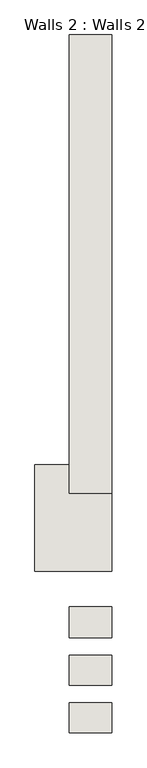
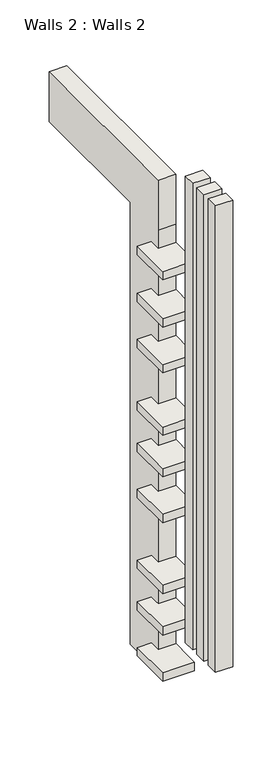
"""IFC4 building model written with IfcOpenShell, lengths in millimetres: wall geometry, Walls 2 : Walls 2."""

from ifc_helpers import new_model, si_unit, frame, origin, place, context, project, spatial, polyline, outline, extrude, source, transform, mapped, element, save


def walls_2_walls_2_6b9d7f67(model_context):
    return source(origin(), model_context, "Body", "SweptSolid", [
        extrude(outline(polyline([(-12336.1369677, -1150.126099), (-12336.1369677, -388.126099), (-11786.2932708, -388.126099), (-11786.2932708, -1150.126099), (-12336.1369677, -1150.126099)])), frame((0.0, 0.0, 9007.4029243), z_axis=(0.0, 0.0, 1.0), x_axis=(1.0, 0.0, 0.0)), (0.0, 0.0, 1.0), 152.4),
        extrude(outline(polyline([(-12336.1369677, -1150.126099), (-12336.1369677, -388.126099), (-11786.2932708, -388.126099), (-11786.2932708, -1150.126099), (-12336.1369677, -1150.126099)])), frame((0.0, 0.0, 8143.8029243), z_axis=(0.0, 0.0, 1.0), x_axis=(1.0, 0.0, 0.0)), (0.0, 0.0, 1.0), 152.4),
        extrude(outline(polyline([(-12336.1369677, -1150.126099), (-12336.1369677, -388.126099), (-11786.2932708, -388.126099), (-11786.2932708, -1150.126099), (-12336.1369677, -1150.126099)])), frame((0.0, 0.0, 7305.6029243), z_axis=(0.0, 0.0, 1.0), x_axis=(1.0, 0.0, 0.0)), (0.0, 0.0, 1.0), 152.4),
        extrude(outline(polyline([(-12336.1369677, -1150.126099), (-12336.1369677, -388.126099), (-11786.2932708, -388.126099), (-11786.2932708, -1150.126099), (-12336.1369677, -1150.126099)])), frame((0.0, 0.0, 6162.6029243), z_axis=(0.0, 0.0, 1.0), x_axis=(1.0, 0.0, 0.0)), (0.0, 0.0, 1.0), 152.4),
        extrude(outline(polyline([(-12336.1369677, -1150.126099), (-12336.1369677, -388.126099), (-11786.2932708, -388.126099), (-11786.2932708, -1150.126099), (-12336.1369677, -1150.126099)])), frame((0.0, 0.0, 5400.6029243), z_axis=(0.0, 0.0, 1.0), x_axis=(1.0, 0.0, 0.0)), (0.0, 0.0, 1.0), 152.4),
        extrude(outline(polyline([(-12336.1369677, -1150.126099), (-12336.1369677, -388.126099), (-11786.2932708, -388.126099), (-11786.2932708, -1150.126099), (-12336.1369677, -1150.126099)])), frame((0.0, 0.0, 4562.4029243), z_axis=(0.0, 0.0, 1.0), x_axis=(1.0, 0.0, 0.0)), (0.0, 0.0, 1.0), 152.4),
        extrude(outline(polyline([(-12336.1369677, -1150.126099), (-12336.1369677, -388.126099), (-11786.2932708, -388.126099), (-11786.2932708, -1150.126099), (-12336.1369677, -1150.126099)])), frame((0.0, 0.0, 3267.0029243), z_axis=(0.0, 0.0, 1.0), x_axis=(1.0, 0.0, 0.0)), (0.0, 0.0, 1.0), 152.4),
        extrude(outline(polyline([(-12336.1369677, -1150.126099), (-12336.1369677, -388.126099), (-11786.2932708, -388.126099), (-11786.2932708, -1150.126099), (-12336.1369677, -1150.126099)])), frame((0.0, 0.0, 2505.0029243), z_axis=(0.0, 0.0, 1.0), x_axis=(1.0, 0.0, 0.0)), (0.0, 0.0, 1.0), 152.4),
        extrude(outline(polyline([(-12336.1369677, -1150.126099), (-12336.1369677, -388.126099), (-11786.2932708, -388.126099), (-11786.2932708, -1150.126099), (-12336.1369677, -1150.126099)])), frame((0.0, 0.0, 1666.8029243), z_axis=(0.0, 0.0, 1.0), x_axis=(1.0, 0.0, 0.0)), (0.0, 0.0, 1.0), 152.4),
        extrude(outline(polyline([(-12091.0932708, -1623.587731), (-12091.0932708, -1404.126099), (-11786.2932708, -1404.126099), (-11786.2932708, -1623.587731), (-12091.0932708, -1623.587731)])), frame((0.0, 0.0, 2438.4), z_axis=(0.0, 0.0, 1.0), x_axis=(1.0, 0.0, 0.0)), (0.0, 0.0, 1.0), 8534.4),
        extrude(outline(polyline([(-12091.0932708, -1962.926099), (-12091.0932708, -1751.0114622), (-11786.2932708, -1751.0114622), (-11786.2932708, -1962.926099), (-12091.0932708, -1962.926099)])), frame((0.0, 0.0, 2438.4), z_axis=(0.0, 0.0, 1.0), x_axis=(1.0, 0.0, 0.0)), (0.0, 0.0, 1.0), 8534.4),
        extrude(outline(polyline([(-12091.0932708, -2304.1326122), (-12091.0932708, -2089.926099), (-11786.2932708, -2089.926099), (-11786.2932708, -2304.1326122), (-12091.0932708, -2304.1326122)])), frame((0.0, 0.0, 2438.4), z_axis=(0.0, 0.0, 1.0), x_axis=(1.0, 0.0, 0.0)), (0.0, 0.0, 1.0), 8534.4),
        extrude(outline(polyline([(-591.326099, 10407.015602), (2680.1483652, 10407.015602), (2680.1483652, 9492.615602), (241.7483652, 9492.615602), (241.7483652, 1415.415602), (-591.326099, 1415.415602), (-591.326099, 9492.615602), (-591.326099, 10407.015602)])), frame((-12091.0932708, 0.0, 0.0), z_axis=(1.0, 0.0, 0.0), x_axis=(0.0, 1.0, 0.0)), (0.0, 0.0, 1.0), 304.8),
    ])


if __name__ == "__main__":
    model = new_model("IFC4")
    model_context = context("Model", 3, world=origin())
    ifc_project = project(units=[si_unit("LENGTHUNIT", "METRE", prefix="MILLI")], contexts=[model_context])
    site = spatial("IfcSite", under=ifc_project)
    building = spatial("IfcBuilding", under=site)
    placement = place(None, origin())
    walls_2_walls_2_shape = walls_2_walls_2_6b9d7f67(model_context)
    element("IfcWall", 1, ObjectType="Walls 2 : Walls 2", at=placement, inside=building, context=model_context, shape_type="MappedRepresentation", body=[
        mapped(walls_2_walls_2_shape, transform((0.0, 0.0, 0.0), x_axis=(1.0, 0.0, 0.0), y_axis=(0.0, 1.0, 0.0), z_axis=(0.0, 0.0, 1.0))),
    ])
    save(model, "model.ifc")

# Revit data of these elements
# Element 1 (IfcWall, "Walls 2 : Walls 2")
#   Materials on its faces: "Default Wall"
# Materials
#   "Default Wall": colour RGB 128 128 128, transparency 0
